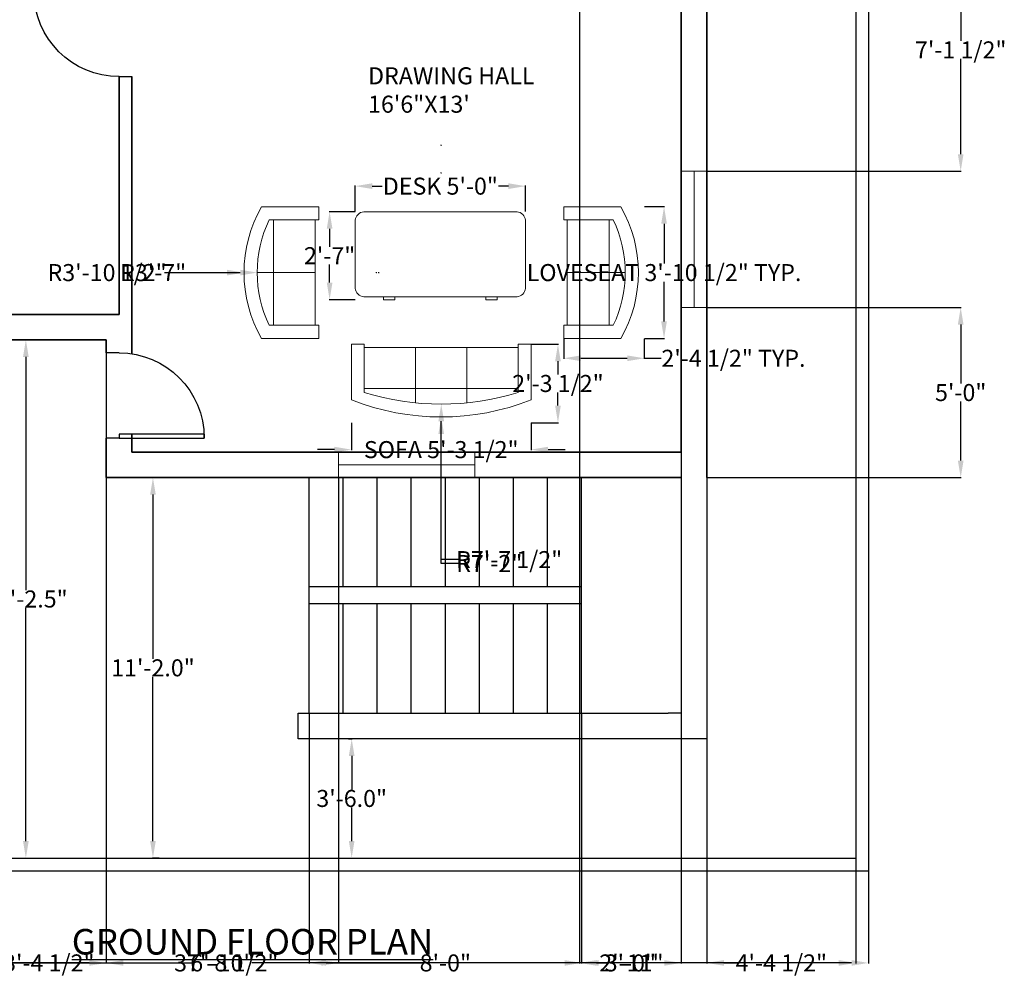
# Model space of a CAD drawing. Units: inches. Extents: x 889 to 1449, y 3224 to 3899.
# Tile 2 of 4: x 1101 to 1448, y 3224 to 3565. Entities that reach past the tile are written whole.
import ezdxf

# ---------------------------------------------------------------- set-up
doc = ezdxf.new("R2010")
doc.units = ezdxf.units.IN
doc.header["$MEASUREMENT"] = 0
for name, color, linetype, lineweight in [('A-ANNO-DIMS', 2, 'Continuous', 18), ('A-ANNO-TEXT', 7, 'Continuous', 25), ('A-AREA-IDEN', 7, 'Continuous', 18), ('A-DOOR', 4, 'Continuous', 25), ('A-FLOR-STRS', 7, 'Continuous', 25), ('A-FURN', 8, 'Continuous', 18), ('A-GLAZ', 4, 'Continuous', 18), ('A-WALL', 7, 'Continuous', 35), ('C-PROP', 7, 'Continuous', 25)]:
    doc.layers.add(name, color=color, linetype=linetype, lineweight=lineweight)
doc.styles.get("Standard").update_dxf_attribs({"font": 'arial.ttf'})
doc.dimstyles.get("Standard").update_dxf_attribs({"dimtxt": 6, "dimasz": 6, "dimexe": 0.18, "dimexo": 0.0625, "dimgap": 0.09, "dimtad": 0, "dimtih": 1, "dimtoh": 1, "dimdec": 1, "dimzin": 0, "dimdsep": 46, "dimlunit": 3, "dimtxsty": 'Standard', "dimcen": 0.09, "dimadec": 0, "dimazin": 0, "dimtfac": 1, "dimtdec": 1, "dimtofl": 0, "dimtmove": 0, "dimatfit": 3, "dimfxl": 1, "dimtolj": 1, "dimtzin": 0, "dimarcsym": 0})

# ---------------------------------------------------------------- blocks, each defined once
blk = doc.blocks.new('*U2')
for p, q in [((0, 0), (0, -6)), ((40, 0), (40, -6))]:
    blk.add_line(p, q)
blk.add_lwpolyline([(0, 0), (0, 40), (1.75, 40), (1.75, 0)], close=True)
blk.add_arc((0, 0), 40, 0, 90)
blk = doc.blocks.new('Sofa - Roundback 7 ft.')
for p, q in [((-12.00002, -32.4421), (-12.00003, -6.5971)), ((11.99997, -32.4421), (11.99998, -6.5971)), ((-36.000027, -34), (-36.000027, -11.4696)), ((-35.999844, -13.3819), (35.9998, -13.3819)), ((35.99998, -34), (35.99998, -11.4696)), ((-36.000027, -32.4421), (35.99998, -32.4421))]:
    blk.add_line(p, q)
for points in [[(-36.000027, -34), (-42.000027, -34), (-42.000027, -8)], [(41.99998, -8), (41.99998, -34), (35.99998, -34)]]:
    blk.add_lwpolyline(points)
for centre, radius, start, end in [((0, -114.25), 114.25, 68.43141, 111.5686), ((-0.00001, -127.1968), 121.1968, 72.72033, 107.2797)]:
    blk.add_arc(centre, radius, start, end)
blk = doc.blocks.new('Sofa - Roundback Loveseat 5 ft.')
for p, q in [((0, -32.44198), (0, -5.99998)), ((-24, -33.99998), (-24, -11.46958)), ((-23.9998, -13.38178), (23.99986, -13.38178)), ((24.00004, -33.99998), (24.00004, -11.46958)), ((-24, -32.44198), (24.00004, -32.44198))]:
    blk.add_line(p, q)
for points in [[(-24, -33.99998), (-30, -33.99998), (-30, -7.99998)], [(30.00004, -7.99998), (30.00004, -33.99998), (24.00004, -33.99998)]]:
    blk.add_lwpolyline(points)
for centre, radius, start, end in [((0, -60.24998), 60.24998, 60.13715, 119.8628), ((0, -61.38438), 55.38444, 64.32083, 115.6792)]:
    blk.add_arc(centre, radius, start, end)
blk = doc.blocks.new('Desk - 30 x 60 in.')
for p, q in [((-26.999995, 0), (26.999995, 0)), ((-29.999995, -27), (-29.999995, -3)), ((29.999995, -3), (29.999995, -27)), ((26.999995, -30), (-26.999995, -30)), ((-20.000005, -30), (-20.000005, -31)), ((-20.000005, -31), (-16.000005, -31)), ((-16.000005, -31), (-16.000005, -30)), ((15.999995, -31), (15.999995, -30)), ((19.999995, -31), (15.999995, -31)), ((19.999995, -30), (19.999995, -31))]:
    blk.add_line(p, q)
for centre, start, end in [((-26.499995, -3.5), 98.1301, 171.8699), ((26.499995, -3.5), 8.130102, 81.8699), ((-26.499995, -26.5), 188.1301, 261.8699), ((26.499995, -26.5), 278.1301, 351.8699)]:
    blk.add_arc(centre, 3.535534, start, end)
blk = doc.blocks.new('*D20')
at = {"layer": 'A-ANNO-DIMS', "color": 0, "lineweight": -2, "transparency": 16777216}
for p, q in [((1150.59, 3403.85), (1148.19, 3403.85)), ((1148.37, 3397.85), (1148.37, 3340.01)), ((1148.37, 3275.85), (1148.37, 3333.7)), ((1150.59, 3269.85), (1148.19, 3269.85))]:
    blk.add_line(p, q, dxfattribs=at)
at = {"layer": 'A-ANNO-DIMS', "color": 0, "transparency": 16777216}
for points in [[(1147.37, 3397.85), (1149.37, 3397.85), (1148.37, 3403.85)], [(1147.37, 3275.85), (1149.37, 3275.85), (1148.37, 3269.85)]]:
    blk.add_solid(points, dxfattribs=at)
at = {"layer": 'Defpoints', "color": 0, "transparency": 16777216}
for p in [(1150.65, 3403.85), (1148.37, 3269.85), (1150.65, 3269.85)]:
    blk.add_point(p, dxfattribs=at)
at = {"layer": 'A-ANNO-DIMS', "color": 0, "transparency": 16777216, "insert": (1148.37, 3336.85), "char_height": 6, "attachment_point": 5}
blk.add_mtext('\\A1;11\'-2.0"', dxfattribs=at)
blk = doc.blocks.new('*D21')
at = {"layer": 'A-ANNO-DIMS', "color": 0, "lineweight": -2, "transparency": 16777216}
for p, q in [((1217.29, 3311.85), (1218.55, 3311.85)), ((1218.37, 3305.85), (1218.37, 3294.01)), ((1218.37, 3275.85), (1218.37, 3287.7)), ((1217.29, 3269.85), (1218.55, 3269.85))]:
    blk.add_line(p, q, dxfattribs=at)
at = {"layer": 'A-ANNO-DIMS', "color": 0, "transparency": 16777216}
for points in [[(1217.37, 3305.85), (1219.37, 3305.85), (1218.37, 3311.85)], [(1217.37, 3275.85), (1219.37, 3275.85), (1218.37, 3269.85)]]:
    blk.add_solid(points, dxfattribs=at)
at = {"layer": 'Defpoints', "color": 0, "transparency": 16777216}
for p in [(1217.23, 3311.85), (1217.23, 3269.85), (1218.37, 3269.85)]:
    blk.add_point(p, dxfattribs=at)
at = {"layer": 'A-ANNO-DIMS', "color": 0, "transparency": 16777216, "insert": (1218.37, 3290.85), "char_height": 6, "attachment_point": 5}
blk.add_mtext('\\A1;3\'-6.0"', dxfattribs=at)
blk = doc.blocks.new('*D22')
at = {"layer": 'A-ANNO-DIMS', "color": 0, "lineweight": -2, "transparency": 16777216}
for p, q in [((1103.67, 3452.35), (1103.79, 3452.35)), ((1103.61, 3446.35), (1103.61, 3364.26)), ((1103.61, 3275.85), (1103.61, 3357.95)), ((1103.67, 3269.85), (1103.79, 3269.85))]:
    blk.add_line(p, q, dxfattribs=at)
at = {"layer": 'A-ANNO-DIMS', "color": 0, "transparency": 16777216}
for points in [[(1102.61, 3446.35), (1104.61, 3446.35), (1103.61, 3452.35)], [(1102.61, 3275.85), (1104.61, 3275.85), (1103.61, 3269.85)]]:
    blk.add_solid(points, dxfattribs=at)
at = {"layer": 'Defpoints', "color": 0, "transparency": 16777216}
for p in [(1103.61, 3452.35), (1103.61, 3269.85), (1103.61, 3269.85)]:
    blk.add_point(p, dxfattribs=at)
at = {"layer": 'A-ANNO-DIMS', "color": 0, "transparency": 16777216, "insert": (1103.61, 3361.1), "char_height": 6, "attachment_point": 5}
blk.add_mtext('\\A1;15\'-2.5"', dxfattribs=at)
blk = doc.blocks.new('WIN-48IN')
blk.add_line((4.5, 48), (4.5, 0))
blk.add_lwpolyline([(9, 48), (9, 0), (0, 0), (0, 48)], close=True)
blk = doc.blocks.new('*D34')
at = {"layer": 'A-ANNO-DIMS', "color": 0, "lineweight": -2, "transparency": 16777216}
for p, q in [((1321.48, 3499.29), (1328.57, 3499.29)), ((1328.39, 3493.29), (1328.39, 3479.27)), ((1328.39, 3458.86), (1328.39, 3472.87)), ((1321.48, 3452.86), (1328.57, 3452.86))]:
    blk.add_line(p, q, dxfattribs=at)
at = {"layer": 'A-ANNO-DIMS', "color": 0, "transparency": 16777216}
for points in [[(1327.39, 3493.29), (1329.39, 3493.29), (1328.39, 3499.29)], [(1327.39, 3458.86), (1329.39, 3458.86), (1328.39, 3452.86)]]:
    blk.add_solid(points, dxfattribs=at)
at = {"layer": 'Defpoints', "color": 0, "transparency": 16777216}
for p in [(1321.42, 3499.29), (1328.39, 3499.29), (1321.42, 3452.86)]:
    blk.add_point(p, dxfattribs=at)
at = {"layer": 'A-ANNO-DIMS', "color": 0, "transparency": 16777216, "insert": (1328.39, 3476.07), "char_height": 6, "attachment_point": 5}
blk.add_mtext('\\A1;LOVESEAT 3\'-10 1/2" TYP.', dxfattribs=at)
blk = doc.blocks.new('*D35')
at = {"layer": 'A-ANNO-DIMS', "color": 0, "lineweight": -2, "transparency": 16777216}
for p, q in [((1293.05, 3452.79), (1293.05, 3445.71)), ((1321.42, 3452.79), (1321.42, 3445.71)), ((1299.05, 3445.89), (1315.42, 3445.89)), ((1321.42, 3445.89), (1327.42, 3445.89))]:
    blk.add_line(p, q, dxfattribs=at)
at = {"layer": 'A-ANNO-DIMS', "color": 0, "transparency": 16777216}
for points in [[(1299.05, 3446.89), (1299.05, 3444.89), (1293.05, 3445.89)], [(1315.42, 3446.89), (1315.42, 3444.89), (1321.42, 3445.89)]]:
    blk.add_solid(points, dxfattribs=at)
at = {"layer": 'Defpoints', "color": 0, "transparency": 16777216}
for p in [(1293.05, 3452.86), (1321.42, 3452.86), (1321.42, 3445.89)]:
    blk.add_point(p, dxfattribs=at)
at = {"layer": 'A-ANNO-DIMS', "color": 0, "transparency": 16777216, "insert": (1352.84, 3445.89), "char_height": 6, "attachment_point": 5}
blk.add_mtext('\\A1;2\'-4 1/2" TYP.', dxfattribs=at)
blk = doc.blocks.new('*D40')
at = {"layer": 'A-ANNO-DIMS', "color": 0, "lineweight": -2, "transparency": 16777216}
for p, q in [((1218.28, 3423.14), (1218.28, 3413.54)), ((1281.53, 3423.14), (1281.53, 3413.54)), ((1212.28, 3413.72), (1206.28, 3413.72)), ((1287.53, 3413.72), (1293.53, 3413.72))]:
    blk.add_line(p, q, dxfattribs=at)
at = {"layer": 'A-ANNO-DIMS', "color": 0, "transparency": 16777216}
for points in [[(1212.28, 3414.72), (1212.28, 3412.72), (1218.28, 3413.72)], [(1287.53, 3414.72), (1287.53, 3412.72), (1281.53, 3413.72)]]:
    blk.add_solid(points, dxfattribs=at)
at = {"layer": 'Defpoints', "color": 0, "transparency": 16777216}
for p in [(1218.28, 3423.2), (1281.53, 3423.2), (1218.28, 3413.72)]:
    blk.add_point(p, dxfattribs=at)
at = {"layer": 'A-ANNO-DIMS', "color": 0, "transparency": 16777216, "insert": (1249.91, 3413.72), "char_height": 6, "attachment_point": 5}
blk.add_mtext('\\A1;SOFA 5\'-3 1/2"', dxfattribs=at)
blk = doc.blocks.new('*D41')
at = {"layer": 'A-ANNO-DIMS', "color": 0, "lineweight": -2, "transparency": 16777216}
for p, q in [((1281.6, 3450.82), (1291.2, 3450.82)), ((1291.02, 3444.82), (1291.02, 3440.2)), ((1291.02, 3429.2), (1291.02, 3433.82)), ((1281.6, 3423.2), (1291.2, 3423.2))]:
    blk.add_line(p, q, dxfattribs=at)
at = {"layer": 'A-ANNO-DIMS', "color": 0, "transparency": 16777216}
for points in [[(1290.02, 3444.82), (1292.02, 3444.82), (1291.02, 3450.82)], [(1290.02, 3429.2), (1292.02, 3429.2), (1291.02, 3423.2)]]:
    blk.add_solid(points, dxfattribs=at)
at = {"layer": 'Defpoints', "color": 0, "transparency": 16777216}
for p in [(1281.53, 3450.82), (1281.53, 3423.2), (1291.02, 3423.2)]:
    blk.add_point(p, dxfattribs=at)
at = {"layer": 'A-ANNO-DIMS', "color": 0, "transparency": 16777216, "insert": (1291.02, 3437.01), "char_height": 6, "attachment_point": 5}
blk.add_mtext('\\A1;2\'-3 1/2"', dxfattribs=at)
blk = doc.blocks.new('*D42')
at = {"layer": 'A-ANNO-DIMS', "color": 0, "lineweight": -2, "transparency": 16777216}
for p, q in [((1219.6, 3497.59), (1219.6, 3506.7)), ((1225.6, 3506.52), (1229.11, 3506.52)), ((1273.6, 3506.52), (1270.1, 3506.52)), ((1279.6, 3497.59), (1279.6, 3506.7))]:
    blk.add_line(p, q, dxfattribs=at)
at = {"layer": 'A-ANNO-DIMS', "color": 0, "transparency": 16777216}
for points in [[(1225.6, 3507.52), (1225.6, 3505.52), (1219.6, 3506.52)], [(1273.6, 3507.52), (1273.6, 3505.52), (1279.6, 3506.52)]]:
    blk.add_solid(points, dxfattribs=at)
at = {"layer": 'Defpoints', "color": 0, "transparency": 16777216}
for p in [(1279.6, 3506.52), (1219.6, 3497.52), (1279.6, 3497.52)]:
    blk.add_point(p, dxfattribs=at)
at = {"layer": 'A-ANNO-DIMS', "color": 0, "transparency": 16777216, "insert": (1249.6, 3506.52), "char_height": 6, "attachment_point": 5}
blk.add_mtext('\\A1;DESK 5\'-0"', dxfattribs=at)
blk = doc.blocks.new('*D43')
at = {"layer": 'A-ANNO-DIMS', "color": 0, "lineweight": -2, "transparency": 16777216}
for p, q in [((1219.54, 3497.52), (1210.42, 3497.52)), ((1210.6, 3491.52), (1210.6, 3485.13)), ((1210.6, 3472.52), (1210.6, 3478.92)), ((1219.54, 3466.52), (1210.42, 3466.52))]:
    blk.add_line(p, q, dxfattribs=at)
at = {"layer": 'A-ANNO-DIMS', "color": 0, "transparency": 16777216}
for points in [[(1209.6, 3491.52), (1211.6, 3491.52), (1210.6, 3497.52)], [(1209.6, 3472.52), (1211.6, 3472.52), (1210.6, 3466.52)]]:
    blk.add_solid(points, dxfattribs=at)
at = {"layer": 'Defpoints', "color": 0, "transparency": 16777216}
for p in [(1210.6, 3497.52), (1219.6, 3497.52), (1219.6, 3466.52)]:
    blk.add_point(p, dxfattribs=at)
at = {"layer": 'A-ANNO-DIMS', "color": 0, "transparency": 16777216, "insert": (1210.6, 3482.02), "char_height": 6, "attachment_point": 5}
blk.add_mtext('\\A1;2\'-7"', dxfattribs=at)
blk = doc.blocks.new('*D44')
at = {"layer": 'A-ANNO-DIMS', "color": 0, "lineweight": -2, "transparency": 16777216}
for p, q in [((947.95, 3265.29), (947.95, 3232.74)), ((1400.45, 3265.29), (1400.45, 3232.74)), ((953.95, 3232.92), (1156.81, 3232.92)), ((1394.45, 3232.92), (1191.58, 3232.92))]:
    blk.add_line(p, q, dxfattribs=at)
at = {"layer": 'A-ANNO-DIMS', "color": 0, "transparency": 16777216}
for points in [[(953.95, 3233.92), (953.95, 3231.92), (947.95, 3232.92)], [(1394.45, 3233.92), (1394.45, 3231.92), (1400.45, 3232.92)]]:
    blk.add_solid(points, dxfattribs=at)
at = {"layer": 'Defpoints', "color": 0, "transparency": 16777216}
for p in [(947.95, 3265.35), (1400.45, 3265.35), (1400.45, 3232.92)]:
    blk.add_point(p, dxfattribs=at)
at = {"layer": 'A-ANNO-DIMS', "color": 0, "transparency": 16777216, "insert": (1174.2, 3232.92), "char_height": 6, "attachment_point": 5}
blk.add_mtext('\\A1;37\'-8 1/2"', dxfattribs=at)
blk = doc.blocks.new('*D45')
at = {"layer": 'A-ANNO-DIMS', "color": 0, "lineweight": -2, "transparency": 16777216}
for p, q in [((1203.36, 3320.79), (1203.36, 3232.74)), ((1299.36, 3320.79), (1299.36, 3232.74)), ((1209.36, 3232.92), (1243.29, 3232.92)), ((1293.36, 3232.92), (1259.43, 3232.92))]:
    blk.add_line(p, q, dxfattribs=at)
at = {"layer": 'A-ANNO-DIMS', "color": 0, "transparency": 16777216}
for points in [[(1209.36, 3233.92), (1209.36, 3231.92), (1203.36, 3232.92)], [(1293.36, 3233.92), (1293.36, 3231.92), (1299.36, 3232.92)]]:
    blk.add_solid(points, dxfattribs=at)
at = {"layer": 'Defpoints', "color": 0, "transparency": 16777216}
for p in [(1203.36, 3320.85), (1299.36, 3320.85), (1299.36, 3232.92)]:
    blk.add_point(p, dxfattribs=at)
at = {"layer": 'A-ANNO-DIMS', "color": 0, "transparency": 16777216, "insert": (1251.36, 3232.92), "char_height": 6, "attachment_point": 5}
blk.add_mtext('\\A1;8\'-0"', dxfattribs=at)
blk = doc.blocks.new('*D46')
at = {"layer": 'A-ANNO-DIMS', "color": 0, "lineweight": -2, "transparency": 16777216}
for p, q in [((1299.36, 3320.79), (1299.36, 3232.74)), ((1334.45, 3320.79), (1334.45, 3232.74)), ((1305.36, 3232.92), (1306.46, 3232.92)), ((1328.45, 3232.92), (1327.35, 3232.92))]:
    blk.add_line(p, q, dxfattribs=at)
at = {"layer": 'A-ANNO-DIMS', "color": 0, "transparency": 16777216}
for points in [[(1305.36, 3233.92), (1305.36, 3231.92), (1299.36, 3232.92)], [(1328.45, 3233.92), (1328.45, 3231.92), (1334.45, 3232.92)]]:
    blk.add_solid(points, dxfattribs=at)
at = {"layer": 'Defpoints', "color": 0, "transparency": 16777216}
for p in [(1299.36, 3320.85), (1334.45, 3320.85), (1334.45, 3232.92)]:
    blk.add_point(p, dxfattribs=at)
at = {"layer": 'A-ANNO-DIMS', "color": 0, "transparency": 16777216, "insert": (1316.9, 3232.92), "char_height": 6, "attachment_point": 5}
blk.add_mtext('\\A1;2\'-11"', dxfattribs=at)
blk = doc.blocks.new('*D47')
at = {"layer": 'A-ANNO-DIMS', "color": 0, "lineweight": -2, "transparency": 16777216}
for p, q in [((1343.45, 3311.79), (1343.45, 3232.74)), ((1395.95, 3269.79), (1395.95, 3232.74)), ((1349.45, 3232.92), (1354.52, 3232.92)), ((1389.95, 3232.92), (1384.87, 3232.92))]:
    blk.add_line(p, q, dxfattribs=at)
at = {"layer": 'A-ANNO-DIMS', "color": 0, "transparency": 16777216}
for points in [[(1349.45, 3233.92), (1349.45, 3231.92), (1343.45, 3232.92)], [(1389.95, 3233.92), (1389.95, 3231.92), (1395.95, 3232.92)]]:
    blk.add_solid(points, dxfattribs=at)
at = {"layer": 'Defpoints', "color": 0, "transparency": 16777216}
for p in [(1343.45, 3311.85), (1395.95, 3269.85), (1395.95, 3232.92)]:
    blk.add_point(p, dxfattribs=at)
at = {"layer": 'A-ANNO-DIMS', "color": 0, "transparency": 16777216, "insert": (1369.7, 3232.92), "char_height": 6, "attachment_point": 5}
blk.add_mtext('\\A1;4\'-4 1/2"', dxfattribs=at)
blk = doc.blocks.new('*D48')
at = {"layer": 'A-ANNO-DIMS', "color": 0, "lineweight": -2, "transparency": 16777216}
for p, q in [((989.45, 3452.29), (989.45, 3232.74)), ((1131.95, 3452.29), (1131.95, 3232.74)), ((995.45, 3232.92), (1041.26, 3232.92)), ((1125.95, 3232.92), (1080.13, 3232.92))]:
    blk.add_line(p, q, dxfattribs=at)
at = {"layer": 'A-ANNO-DIMS', "color": 0, "transparency": 16777216}
for points in [[(995.45, 3233.92), (995.45, 3231.92), (989.45, 3232.92)], [(1125.95, 3233.92), (1125.95, 3231.92), (1131.95, 3232.92)]]:
    blk.add_solid(points, dxfattribs=at)
at = {"layer": 'Defpoints', "color": 0, "transparency": 16777216}
for p in [(989.45, 3452.35), (1131.95, 3452.35), (1131.95, 3232.92)]:
    blk.add_point(p, dxfattribs=at)
at = {"layer": 'A-ANNO-DIMS', "color": 0, "transparency": 16777216, "insert": (1060.7, 3232.92), "char_height": 6, "attachment_point": 5}
blk.add_mtext('\\A1;11\'-10 1/2"', dxfattribs=at)
blk = doc.blocks.new('*D50')
at = {"layer": 'A-ANNO-DIMS', "color": 0, "lineweight": -2, "transparency": 16777216}
for p, q in [((1343.51, 3463.78), (1433.06, 3463.78)), ((1432.88, 3457.78), (1432.88, 3436.97)), ((1432.88, 3409.85), (1432.88, 3430.66)), ((1343.51, 3403.85), (1433.06, 3403.85))]:
    blk.add_line(p, q, dxfattribs=at)
at = {"layer": 'A-ANNO-DIMS', "color": 0, "transparency": 16777216}
for points in [[(1431.88, 3457.78), (1433.88, 3457.78), (1432.88, 3463.78)], [(1431.88, 3409.85), (1433.88, 3409.85), (1432.88, 3403.85)]]:
    blk.add_solid(points, dxfattribs=at)
at = {"layer": 'Defpoints', "color": 0, "transparency": 16777216}
for p in [(1343.45, 3463.78), (1432.88, 3463.78), (1343.45, 3403.85)]:
    blk.add_point(p, dxfattribs=at)
at = {"layer": 'A-ANNO-DIMS', "color": 0, "transparency": 16777216, "insert": (1432.88, 3433.82), "char_height": 6, "attachment_point": 5}
blk.add_mtext('\\A1;5\'-0"', dxfattribs=at)
blk = doc.blocks.new('*D51')
at = {"layer": 'A-ANNO-DIMS', "color": 0, "lineweight": -2, "transparency": 16777216}
for p, q in [((1343.51, 3597.24), (1433.06, 3597.24)), ((1432.88, 3591.24), (1432.88, 3557.7)), ((1432.88, 3517.78), (1432.88, 3551.32)), ((1343.51, 3511.78), (1433.06, 3511.78))]:
    blk.add_line(p, q, dxfattribs=at)
at = {"layer": 'A-ANNO-DIMS', "color": 0, "transparency": 16777216}
for points in [[(1431.88, 3591.24), (1433.88, 3591.24), (1432.88, 3597.24)], [(1431.88, 3517.78), (1433.88, 3517.78), (1432.88, 3511.78)]]:
    blk.add_solid(points, dxfattribs=at)
at = {"layer": 'Defpoints', "color": 0, "transparency": 16777216}
for p in [(1343.45, 3597.24), (1432.88, 3597.24), (1343.45, 3511.78)]:
    blk.add_point(p, dxfattribs=at)
at = {"layer": 'A-ANNO-DIMS', "color": 0, "transparency": 16777216, "insert": (1432.88, 3554.51), "char_height": 6, "attachment_point": 5}
blk.add_mtext('\\A1;7\'-1 1/2"', dxfattribs=at)
blk = doc.blocks.new('*D56')
at = {"layer": 'A-ANNO-DIMS', "color": 0, "lineweight": -2, "transparency": 16777216}
for p, q in [((1131.95, 3403.79), (1131.95, 3232.74)), ((1213.7, 3403.79), (1213.7, 3232.74)), ((1137.95, 3232.92), (1162.41, 3232.92)), ((1207.7, 3232.92), (1183.23, 3232.92))]:
    blk.add_line(p, q, dxfattribs=at)
at = {"layer": 'A-ANNO-DIMS', "color": 0, "transparency": 16777216}
for points in [[(1137.95, 3233.92), (1137.95, 3231.92), (1131.95, 3232.92)], [(1207.7, 3233.92), (1207.7, 3231.92), (1213.7, 3232.92)]]:
    blk.add_solid(points, dxfattribs=at)
at = {"layer": 'Defpoints', "color": 0, "transparency": 16777216}
for p in [(1131.95, 3403.85), (1213.7, 3403.85), (1213.7, 3232.92)]:
    blk.add_point(p, dxfattribs=at)
at = {"layer": 'A-ANNO-DIMS', "color": 0, "transparency": 16777216, "insert": (1172.82, 3232.92), "char_height": 6, "attachment_point": 5}
blk.add_mtext('\\A1;6\'-10"', dxfattribs=at)
blk = doc.blocks.new('*D57')
at = {"layer": 'A-ANNO-DIMS', "color": 0, "lineweight": -2, "transparency": 16777216}
for p, q in [((1091.445734, 3452.292373), (1091.445734, 3232.744873)), ((1131.945734, 3452.292373), (1131.945734, 3232.744873)), ((1085.445734, 3232.924873), (1079.445734, 3232.924873)), ((1137.945734, 3232.924873), (1143.945734, 3232.924873))]:
    blk.add_line(p, q, dxfattribs=at)
at = {"layer": 'A-ANNO-DIMS', "color": 0, "transparency": 16777216}
for points in [[(1085.445734, 3233.924873), (1085.445734, 3231.924873), (1091.445734, 3232.924873)], [(1137.945734, 3233.924873), (1137.945734, 3231.924873), (1131.945734, 3232.924873)]]:
    blk.add_solid(points, dxfattribs=at)
at = {"layer": 'Defpoints', "color": 0, "transparency": 16777216}
for p in [(1091.445734, 3452.354873), (1131.945734, 3452.354873), (1131.945734, 3232.924873)]:
    blk.add_point(p, dxfattribs=at)
at = {"layer": 'A-ANNO-DIMS', "color": 0, "transparency": 16777216, "insert": (1111.695734, 3232.924873), "char_height": 6, "attachment_point": 5}
blk.add_mtext('\\A1;3\'-4 1/2"', dxfattribs=at)
blk = doc.blocks.new('*D60')
at = {"layer": 'A-ANNO-DIMS', "color": 0, "lineweight": -2, "transparency": 16777216}
for p, q in [((1298.62, 3661.08), (1298.62, 3232.74)), ((1334.45, 3661.08), (1334.45, 3232.74)), ((1304.62, 3232.92), (1308.47, 3232.92)), ((1328.45, 3232.92), (1324.6, 3232.92))]:
    blk.add_line(p, q, dxfattribs=at)
at = {"layer": 'A-ANNO-DIMS', "color": 0, "transparency": 16777216}
for points in [[(1304.62, 3233.92), (1304.62, 3231.92), (1298.62, 3232.92)], [(1328.45, 3233.92), (1328.45, 3231.92), (1334.45, 3232.92)]]:
    blk.add_solid(points, dxfattribs=at)
at = {"layer": 'Defpoints', "color": 0, "transparency": 16777216}
for p in [(1298.62, 3661.14), (1334.45, 3661.14), (1334.45, 3232.92)]:
    blk.add_point(p, dxfattribs=at)
at = {"layer": 'A-ANNO-DIMS', "color": 0, "transparency": 16777216, "insert": (1316.53, 3232.92), "char_height": 6, "attachment_point": 5}
blk.add_mtext('\\A1;3\'-0"', dxfattribs=at)
blk = doc.blocks.new('*D65')
at = {"layer": 'A-ANNO-DIMS', "color": 0, "lineweight": -2, "transparency": 16777216}
for p, q in [((1249.82, 3521), (1250, 3521)), ((1249.91, 3520.91), (1249.91, 3521.09)), ((1249.91, 3374.97), (1249.91, 3423.73)), ((1255.91, 3374.97), (1249.91, 3374.97))]:
    blk.add_line(p, q, dxfattribs=at)
at = {"layer": 'A-ANNO-DIMS', "color": 0, "transparency": 16777216}
blk.add_solid([(1250.91, 3423.73), (1248.91, 3423.73), (1249.91, 3429.73)], dxfattribs=at)
at = {"layer": 'Defpoints', "color": 0, "transparency": 16777216}
for p in [(1249.91, 3521), (1249.91, 3429.73)]:
    blk.add_point(p, dxfattribs=at)
at = {"layer": 'A-ANNO-DIMS', "color": 0, "transparency": 16777216, "insert": (1273.83, 3374.97), "char_height": 6, "attachment_point": 5}
blk.add_mtext('\\A1;R7\'-7 1/2"', dxfattribs=at)
blk = doc.blocks.new('*D66')
at = {"layer": 'A-ANNO-DIMS', "color": 0, "lineweight": -2, "transparency": 16777216}
for p, q in [((1249.82, 3511.25), (1250, 3511.25)), ((1249.91, 3511.16), (1249.91, 3511.34)), ((1249.91, 3373.59), (1249.91, 3419.21)), ((1255.91, 3373.59), (1249.91, 3373.59))]:
    blk.add_line(p, q, dxfattribs=at)
at = {"layer": 'A-ANNO-DIMS', "color": 0, "transparency": 16777216}
blk.add_solid([(1250.91, 3419.21), (1248.91, 3419.21), (1249.91, 3425.21)], dxfattribs=at)
at = {"layer": 'Defpoints', "color": 0, "transparency": 16777216}
for p in [(1249.91, 3511.25), (1249.91, 3425.21)]:
    blk.add_point(p, dxfattribs=at)
at = {"layer": 'A-ANNO-DIMS', "color": 0, "transparency": 16777216, "insert": (1266.84, 3373.59), "char_height": 6, "attachment_point": 5}
blk.add_mtext('\\A1;R7\'-2"', dxfattribs=at)
blk = doc.blocks.new('*D67')
at = {"layer": 'A-ANNO-DIMS', "color": 0, "lineweight": -2, "transparency": 16777216}
for p, q in [((1152.48, 3476.07), (1174.45, 3476.07)), ((1226.99, 3476.07), (1227.17, 3476.07)), ((1227.08, 3475.98), (1227.08, 3476.16))]:
    blk.add_line(p, q, dxfattribs=at)
at = {"layer": 'A-ANNO-DIMS', "color": 0, "transparency": 16777216}
blk.add_solid([(1174.45, 3477.07), (1174.45, 3475.07), (1180.45, 3476.07)], dxfattribs=at)
at = {"layer": 'Defpoints', "color": 0, "transparency": 16777216}
for p in [(1180.45, 3476.07), (1227.08, 3476.07)]:
    blk.add_point(p, dxfattribs=at)
at = {"layer": 'A-ANNO-DIMS', "color": 0, "transparency": 16777216, "insert": (1132.22, 3476.07), "char_height": 6, "attachment_point": 5}
blk.add_mtext('\\A1;R3\'-10 1/2"', dxfattribs=at)
blk = doc.blocks.new('*D68')
at = {"layer": 'A-ANNO-DIMS', "color": 0, "lineweight": -2, "transparency": 16777216}
for p, q in [((1159.38, 3476.07), (1179.1, 3476.07)), ((1227.87, 3476.07), (1228.05, 3476.07)), ((1227.96, 3475.98), (1227.96, 3476.16))]:
    blk.add_line(p, q, dxfattribs=at)
at = {"layer": 'A-ANNO-DIMS', "color": 0, "transparency": 16777216}
blk.add_solid([(1179.1, 3477.07), (1179.1, 3475.07), (1185.1, 3476.07)], dxfattribs=at)
at = {"layer": 'Defpoints', "color": 0, "transparency": 16777216}
for p in [(1185.1, 3476.07), (1227.96, 3476.07)]:
    blk.add_point(p, dxfattribs=at)
at = {"layer": 'A-ANNO-DIMS', "color": 0, "transparency": 16777216, "insert": (1148.45, 3476.07), "char_height": 6, "attachment_point": 5}
blk.add_mtext('\\A1;R3\'-7"', dxfattribs=at)

msp = doc.modelspace()

# ---------------------------------------------------------------- linework, layer by layer
at = {"layer": 'A-FLOR-STRS'}
for p, q in [((1203.36, 3320.85), (1203.36, 3403.85)), ((1215.36, 3365.35), (1215.36, 3403.85)), ((1227.36, 3365.35), (1227.36, 3403.85)), ((1239.36, 3365.35), (1239.36, 3403.85)), ((1251.36, 3365.35), (1251.36, 3403.85)), ((1263.36, 3365.35), (1263.36, 3403.85)), ((1275.36, 3365.35), (1275.36, 3403.85)), ((1287.36, 3365.35), (1287.36, 3403.85)), ((1299.36, 3320.85), (1299.36, 3403.85)), ((1334.45, 3403.85), (1334.45, 3320.85)), ((1343.45, 3403.85), (1343.45, 3311.85)), ((1299.36, 3365.35), (1203.36, 3365.35)), ((1299.36, 3359.35), (1203.36, 3359.35)), ((1215.36, 3320.85), (1215.36, 3359.35)), ((1227.36, 3320.85), (1227.36, 3359.35)), ((1239.36, 3320.85), (1239.36, 3359.35)), ((1251.36, 3320.85), (1251.36, 3359.35)), ((1263.36, 3320.85), (1263.36, 3359.35)), ((1275.36, 3320.85), (1275.36, 3359.35)), ((1287.36, 3320.85), (1287.36, 3359.35)), ((1199.58, 3311.85), (1199.58, 3320.85)), ((1199.58, 3320.85), (1329.79, 3320.85)), ((1334.45, 3320.85), (1329.79, 3320.85)), ((1343.45, 3311.85), (1199.58, 3311.85))]:
    msp.add_line(p, q, dxfattribs=at)
at = {"layer": 'A-WALL'}
for p, q in [((1343.45, 3674.35), (1343.45, 3403.85)), ((1334.45, 3568.85), (1334.45, 3412.85)), ((1136.45, 3545.09), (1136.45, 3461.35)), ((1140.95, 3545.09), (1140.95, 3447.45)), ((998.45, 3461.35), (1136.45, 3461.35)), ((989.45, 3452.35), (1131.95, 3452.35)), ((1131.95, 3452.35), (1131.95, 3447.79)), ((1131.95, 3417.79), (1131.95, 3403.85)), ((1140.95, 3419.1), (1140.95, 3412.85)), ((1140.95, 3412.85), (1334.45, 3412.85)), ((1131.95, 3403.85), (1334.45, 3403.85))]:
    msp.add_line(p, q, dxfattribs=at)
at = {"layer": 'C-PROP'}
for p, q in [((1400.45, 3857.35), (1400.45, 3265.35)), ((1395.95, 3750.85), (1395.95, 3269.85)), ((952.45, 3269.85), (1395.95, 3269.85)), ((947.95, 3265.35), (1400.45, 3265.35))]:
    msp.add_line(p, q, dxfattribs=at)

# ---------------------------------------------------------------- block references
at = {"layer": 'A-DOOR', "xscale": -0.75, "yscale": 0.75, "zscale": 0.75}
for p, rotation in [((1136.45, 3575.09), 90), ((1136.45, 3417.79), 270)]:
    msp.add_blockref('*U2', p, dxfattribs=dict(at, rotation=rotation))
at = {"layer": 'A-FURN'}
for name, p, xscale, yscale, zscale, rotation in [('Sofa - Roundback Loveseat 5 ft.', (1180.45, 3476.07), 0.7738497298971354, 0.7738497298971354, 0.7738497298971354, 90), ('Sofa - Roundback Loveseat 5 ft.', (1319.36, 3476.07), -0.7738497298971354, 0.7738497298971354, 0.7738497298971354, 270), ('Sofa - Roundback 7 ft.', (1249.91, 3425.21), 0.7530480268685884, 0.7530480268685884, 0.7530480268685884, 180)]:
    msp.add_blockref(name, p, dxfattribs=dict(at, xscale=xscale, yscale=yscale, zscale=zscale, rotation=rotation))
msp.add_blockref('Desk - 30 x 60 in.', (1249.6, 3497.52), dxfattribs=at)
at = {"layer": 'A-GLAZ'}
msp.add_blockref('WIN-48IN', (1334.45, 3463.78), dxfattribs=at)
at = {"layer": 'A-GLAZ', "rotation": 90.00000000000063}
msp.add_blockref('WIN-48IN', (1261.7, 3403.86), dxfattribs=at)

# ---------------------------------------------------------------- texts
at = {"layer": 'A-ANNO-TEXT', "insert": (1119.78, 3244.88), "char_height": 9, "attachment_point": 1}
msp.add_mtext_dynamic_manual_height_columns('{\\fArial|b1|i0|c0|p34;\\LGROUND FLOOR PLAN}', width=396.8668, gutter_width=1, heights=[0], dxfattribs=at)
at = {"layer": 'A-AREA-IDEN', "insert": (1224.14, 3548.38), "char_height": 6, "attachment_point": 1}
msp.add_mtext_dynamic_manual_height_columns('DRAWING HALL\\P16\'6"X13\'', width=93.4406, gutter_width=1, heights=[0], dxfattribs=at)

# ---------------------------------------------------------------- dimensions: what is measured, and where the dimension line sits
at = {"layer": 'A-ANNO-DIMS'}
for base, p1, p2, picture, middle in [((1334.45, 3232.92), (1298.62, 3661.14), (1334.45, 3661.14), '*D60', (1316.53, 3232.92)), ((1131.95, 3232.92), (989.45, 3452.35), (1131.95, 3452.35), '*D48', (1060.7, 3232.92)), ((1131.95, 3232.92), (1091.45, 3452.35), (1131.95, 3452.35), '*D57', (1111.7, 3232.92)), ((1213.695734, 3232.924873), (1131.945734, 3403.854873), (1213.695734, 3403.854873), '*D56', (1172.820734, 3232.924873)), ((1299.36, 3232.92), (1203.36, 3320.85), (1299.36, 3320.85), '*D45', (1251.36, 3232.92)), ((1334.45, 3232.92), (1299.36, 3320.85), (1334.45, 3320.85), '*D46', (1316.9, 3232.92)), ((1395.95, 3232.92), (1343.45, 3311.85), (1395.95, 3269.85), '*D47', (1369.7, 3232.92)), ((1400.45, 3232.92), (947.95, 3265.35), (1400.45, 3265.35), '*D44', (1174.2, 3232.92))]:
    dim = msp.add_linear_dim(base=base, p1=p1, p2=p2, dimstyle='Standard', override={"dimdec": 1, "dimlfac": 1, "dimrnd": 0, "dimzin": 1, "dimdsep": 46, "dimlunit": 4, "dimfrac": 2}, dxfattribs=at)
    dim.commit()
    dim.dimension.update_dxf_attribs({"geometry": picture, "text_midpoint": middle})
for base, p1, p2, angle, override, picture, middle in [((1432.88, 3597.24), (1343.45, 3511.78), (1343.45, 3597.24), 90, {"dimdec": 1, "dimlfac": 1, "dimrnd": 0, "dimzin": 1, "dimdsep": 46, "dimlunit": 4, "dimfrac": 2}, '*D51', (1432.88, 3554.51)), ((1210.6, 3497.52), (1219.6, 3466.52), (1219.6, 3497.52), 90, {"dimdec": 1, "dimlfac": 1, "dimrnd": 0, "dimzin": 1, "dimdsep": 46, "dimlunit": 4, "dimfrac": 2}, '*D43', (1210.6, 3482.02)), ((1432.88, 3463.78), (1343.45, 3403.85), (1343.45, 3463.78), 90, {"dimdec": 1, "dimlfac": 1, "dimrnd": 0, "dimzin": 1, "dimdsep": 46, "dimlunit": 4, "dimfrac": 2}, '*D50', (1432.88, 3433.82)), ((1103.61, 3269.85), (1103.61, 3452.35), (1103.61, 3269.85), 90, {"dimclrd": 0, "dimclre": 0, "dimclrt": 0}, '*D22', (1103.61, 3361.1)), ((1291.02, 3423.2), (1281.53, 3450.82), (1281.53, 3423.2), 270, {"dimdec": 1, "dimlfac": 1, "dimrnd": 0, "dimzin": 1, "dimdsep": 46, "dimlunit": 4, "dimfrac": 2}, '*D41', (1291.02, 3437.01)), ((1148.37, 3269.85), (1150.65, 3403.85), (1150.65, 3269.85), 90, {"dimclrd": 0, "dimclre": 0, "dimclrt": 0}, '*D20', (1148.37, 3336.85)), ((1218.37, 3269.85), (1217.23, 3311.85), (1217.23, 3269.85), 90, {"dimclrd": 0, "dimclre": 0, "dimclrt": 0}, '*D21', (1218.37, 3290.85))]:
    dim = msp.add_linear_dim(base=base, p1=p1, p2=p2, angle=angle, dimstyle='Standard', override=override, dxfattribs=at)
    dim.commit()
    dim.dimension.update_dxf_attribs({"geometry": picture, "text_midpoint": middle})
for center, mpoint, picture, middle in [((1249.91, 3521), (1249.91, 3429.73), '*D65', (1273.83, 3374.97)), ((1249.91, 3511.25), (1249.91, 3425.21), '*D66', (1266.84, 3373.59)), ((1227.08, 3476.07), (1180.45, 3476.07), '*D67', (1152.48, 3476.07)), ((1227.96, 3476.07), (1185.1, 3476.07), '*D68', (1159.38, 3476.07))]:
    dim = msp.add_radius_dim(center=center, mpoint=mpoint, dimstyle='Standard', override={"dimdec": 1, "dimlfac": 1, "dimrnd": 0, "dimzin": 1, "dimdsep": 46, "dimlunit": 4, "dimfrac": 2}, dxfattribs=at)
    dim.commit()
    dim.dimension.update_dxf_attribs({"geometry": picture, "text_midpoint": middle, "dimtype": 164})
for base, p1, p2, text, picture, middle in [((1279.6, 3506.52), (1219.6, 3497.52), (1279.6, 3497.52), 'DESK <>', '*D42', (1249.6, 3506.52)), ((1321.42, 3445.89), (1293.05, 3452.86), (1321.42, 3452.86), '<> TYP.', '*D35', (1352.84, 3445.89))]:
    dim = msp.add_linear_dim(base=base, p1=p1, p2=p2, text=text, dimstyle='Standard', override={"dimdec": 1, "dimlfac": 1, "dimrnd": 0, "dimzin": 1, "dimdsep": 46, "dimlunit": 4, "dimfrac": 2}, dxfattribs=at)
    dim.commit()
    dim.dimension.update_dxf_attribs({"geometry": picture, "text_midpoint": middle})
for base, p1, p2, angle, text, picture, middle in [((1328.39, 3499.29), (1321.42, 3452.86), (1321.42, 3499.29), 90, 'LOVESEAT <> TYP.', '*D34', (1328.39, 3476.07)), ((1218.2777, 3413.7162), (1281.5337, 3423.2046), (1218.2777, 3423.2046), 180, 'SOFA <>', '*D40', (1249.9057, 3413.7162))]:
    dim = msp.add_linear_dim(base=base, p1=p1, p2=p2, angle=angle, text=text, dimstyle='Standard', override={"dimdec": 1, "dimlfac": 1, "dimrnd": 0, "dimzin": 1, "dimdsep": 46, "dimlunit": 4, "dimfrac": 2}, dxfattribs=at)
    dim.commit()
    dim.dimension.update_dxf_attribs({"geometry": picture, "text_midpoint": middle})

doc.saveas('drawing.dxf')
